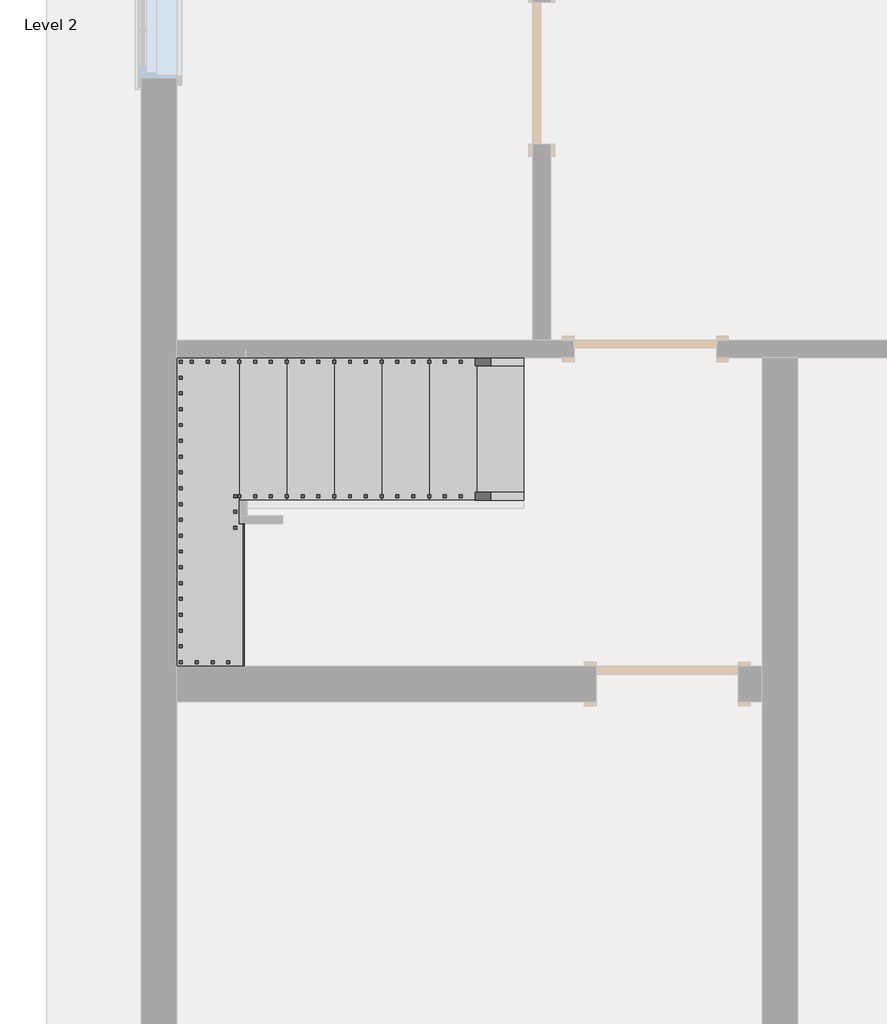
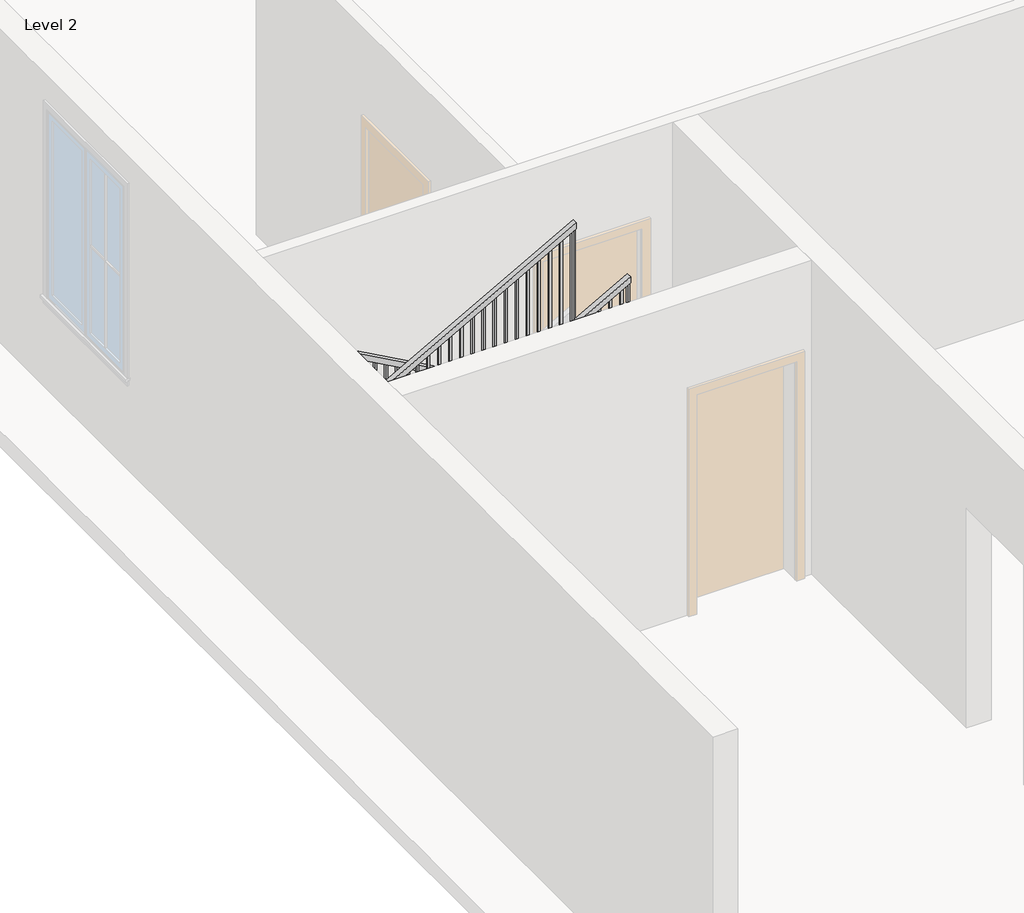
# One storey, part 2 of 3: 2 railings, 1 stair flight.
"""IFC4 building model written with IfcOpenShell, lengths in millimetres."""

from ifc_helpers import new_model, si_unit, frame, origin, place, context, project, spatial, polyline, outline, extrude, faceted_brep, transform, mapped, element, save
from components import stair_flight_2ee17b95

model = new_model("IFC4")

# Units and contexts
model_context = context("Model", 3, world=origin())
ifc_project = project(units=[si_unit("LENGTHUNIT", "METRE", prefix="MILLI")], contexts=[model_context])

# Site, building, storey
site = spatial("IfcSite", under=ifc_project)
building = spatial("IfcBuilding", under=site)
storey = spatial("IfcBuildingStorey", under=building, Name="Level 2", Elevation=3048.0)

# Railings
placement = place(None, origin())
element("IfcRailing", 1, ObjectType="Handrail - Rectangular", at=placement, inside=storey, context=model_context, shape_type="SolidModel", body=[
    faceted_brep([(3727.9146873, 3657.6, 4131.7333333), (3727.9146873, 3657.6, 4073.620221), (3727.9146873, 3708.4, 4073.620221), (3727.9146873, 3708.4, 4131.7333333), (1899.1146873, 3657.6, 5147.7333333), (1885.9510851, 3657.6, 5096.9333333), (1885.9510851, 3708.4, 5096.9333333), (1899.1146873, 3708.4, 5147.7333333), (1549.4, 3657.6, 5147.7333333), (1549.4, 3657.6, 5096.9333333), (1498.6, 3708.4, 5096.9333333), (1498.6, 3708.4, 5147.7333333), (1549.4, 1778.0, 5147.7333333), (1549.4, 1778.0, 5096.9333333), (1498.6, 1727.2, 5096.9333333), (1498.6, 1727.2, 5147.7333333), (1594.3146873, 1778.0, 5147.7333333), (1607.4782895, 1778.0, 5096.9333333), (1607.4782895, 1727.2, 5096.9333333), (1594.3146873, 1727.2, 5147.7333333), (3727.9146873, 1778.0, 6333.0666667), (3727.9146873, 1727.2, 6333.0666667), (3727.9146873, 1727.2, 6274.9535543), (3727.9146873, 1778.0, 6274.9535543)], [[[0, 1, 2, 3]], [[1, 0, 4, 5]], [[2, 1, 5, 6]], [[3, 2, 6, 7]], [[0, 3, 7, 4]], [[5, 4, 8, 9]], [[6, 5, 9, 10]], [[7, 6, 10, 11]], [[4, 7, 11, 8]], [[9, 8, 12, 13]], [[10, 9, 13, 14]], [[11, 10, 14, 15]], [[8, 11, 15, 12]], [[13, 12, 16, 17]], [[14, 13, 17, 18]], [[15, 14, 18, 19]], [[12, 15, 19, 16]], [[20, 21, 22, 23]], [[17, 16, 20, 23]], [[18, 17, 23, 22]], [[19, 18, 22, 21]], [[16, 19, 21, 20]]]),
    extrude(outline(polyline([(6241.1815058, 3667.125), (6230.5981725, 3648.075), (5249.3333333, 3648.075), (5249.3333333, 3667.125), (6241.1815058, 3667.125)])), frame((0.0, 1743.075, 0.0), z_axis=(0.0, 1.0, 0.0), x_axis=(0.0, 0.0, 1.0)), (0.0, 0.0, 1.0), 19.05),
    extrude(outline(polyline([(6184.7370614, 3565.525), (6174.153728, 3546.475), (5249.3333333, 3546.475), (5249.3333333, 3565.525), (6184.7370614, 3565.525)])), frame((0.0, 1743.075, 0.0), z_axis=(0.0, 1.0, 0.0), x_axis=(0.0, 0.0, 1.0)), (0.0, 0.0, 1.0), 19.05),
    extrude(outline(polyline([(6128.2926169, 3463.925), (6117.7092836, 3444.875), (5249.3333333, 3444.875), (5249.3333333, 3463.925), (6128.2926169, 3463.925)])), frame((0.0, 1743.075, 0.0), z_axis=(0.0, 1.0, 0.0), x_axis=(0.0, 0.0, 1.0)), (0.0, 0.0, 1.0), 19.05),
    extrude(outline(polyline([(6071.8481725, 3362.325), (6061.2648391, 3343.275), (5080.0, 3343.275), (5080.0, 3362.325), (6071.8481725, 3362.325)])), frame((0.0, 1743.075, 0.0), z_axis=(0.0, 1.0, 0.0), x_axis=(0.0, 0.0, 1.0)), (0.0, 0.0, 1.0), 19.05),
    extrude(outline(polyline([(6015.403728, 3260.725), (6004.8203947, 3241.675), (5080.0, 3241.675), (5080.0, 3260.725), (6015.403728, 3260.725)])), frame((0.0, 1743.075, 0.0), z_axis=(0.0, 1.0, 0.0), x_axis=(0.0, 0.0, 1.0)), (0.0, 0.0, 1.0), 19.05),
    extrude(outline(polyline([(5958.9592836, 3159.125), (5948.3759503, 3140.075), (5080.0, 3140.075), (5080.0, 3159.125), (5958.9592836, 3159.125)])), frame((0.0, 1743.075, 0.0), z_axis=(0.0, 1.0, 0.0), x_axis=(0.0, 0.0, 1.0)), (0.0, 0.0, 1.0), 19.05),
    extrude(outline(polyline([(5902.5148391, 3057.525), (5891.9315058, 3038.475), (4910.6666667, 3038.475), (4910.6666667, 3057.525), (5902.5148391, 3057.525)])), frame((0.0, 1743.075, 0.0), z_axis=(0.0, 1.0, 0.0), x_axis=(0.0, 0.0, 1.0)), (0.0, 0.0, 1.0), 19.05),
    extrude(outline(polyline([(5846.0703947, 2955.925), (5835.4870614, 2936.875), (4910.6666667, 2936.875), (4910.6666667, 2955.925), (5846.0703947, 2955.925)])), frame((0.0, 1743.075, 0.0), z_axis=(0.0, 1.0, 0.0), x_axis=(0.0, 0.0, 1.0)), (0.0, 0.0, 1.0), 19.05),
    extrude(outline(polyline([(5789.6259503, 2854.325), (5779.0426169, 2835.275), (4910.6666667, 2835.275), (4910.6666667, 2854.325), (5789.6259503, 2854.325)])), frame((0.0, 1743.075, 0.0), z_axis=(0.0, 1.0, 0.0), x_axis=(0.0, 0.0, 1.0)), (0.0, 0.0, 1.0), 19.05),
    extrude(outline(polyline([(5733.1815058, 2752.725), (5722.5981725, 2733.675), (4741.3333333, 2733.675), (4741.3333333, 2752.725), (5733.1815058, 2752.725)])), frame((0.0, 1743.075, 0.0), z_axis=(0.0, 1.0, 0.0), x_axis=(0.0, 0.0, 1.0)), (0.0, 0.0, 1.0), 19.05),
    extrude(outline(polyline([(5676.7370614, 2651.125), (5666.153728, 2632.075), (4741.3333333, 2632.075), (4741.3333333, 2651.125), (5676.7370614, 2651.125)])), frame((0.0, 1743.075, 0.0), z_axis=(0.0, 1.0, 0.0), x_axis=(0.0, 0.0, 1.0)), (0.0, 0.0, 1.0), 19.05),
    extrude(outline(polyline([(5620.2926169, 2549.525), (5609.7092836, 2530.475), (4741.3333333, 2530.475), (4741.3333333, 2549.525), (5620.2926169, 2549.525)])), frame((0.0, 1743.075, 0.0), z_axis=(0.0, 1.0, 0.0), x_axis=(0.0, 0.0, 1.0)), (0.0, 0.0, 1.0), 19.05),
    extrude(outline(polyline([(5563.8481725, 2447.925), (5553.2648391, 2428.875), (4572.0, 2428.875), (4572.0, 2447.925), (5563.8481725, 2447.925)])), frame((0.0, 1743.075, 0.0), z_axis=(0.0, 1.0, 0.0), x_axis=(0.0, 0.0, 1.0)), (0.0, 0.0, 1.0), 19.05),
    extrude(outline(polyline([(5507.403728, 2346.325), (5496.8203947, 2327.275), (4572.0, 2327.275), (4572.0, 2346.325), (5507.403728, 2346.325)])), frame((0.0, 1743.075, 0.0), z_axis=(0.0, 1.0, 0.0), x_axis=(0.0, 0.0, 1.0)), (0.0, 0.0, 1.0), 19.05),
    extrude(outline(polyline([(5450.9592836, 2244.725), (5440.3759503, 2225.675), (4572.0, 2225.675), (4572.0, 2244.725), (5450.9592836, 2244.725)])), frame((0.0, 1743.075, 0.0), z_axis=(0.0, 1.0, 0.0), x_axis=(0.0, 0.0, 1.0)), (0.0, 0.0, 1.0), 19.05),
    extrude(outline(polyline([(5394.5148391, 2143.125), (5383.9315058, 2124.075), (4402.6666667, 2124.075), (4402.6666667, 2143.125), (5394.5148391, 2143.125)])), frame((0.0, 1743.075, 0.0), z_axis=(0.0, 1.0, 0.0), x_axis=(0.0, 0.0, 1.0)), (0.0, 0.0, 1.0), 19.05),
    extrude(outline(polyline([(5338.0703947, 2041.525), (5327.4870614, 2022.475), (4402.6666667, 2022.475), (4402.6666667, 2041.525), (5338.0703947, 2041.525)])), frame((0.0, 1743.075, 0.0), z_axis=(0.0, 1.0, 0.0), x_axis=(0.0, 0.0, 1.0)), (0.0, 0.0, 1.0), 19.05),
    extrude(outline(polyline([(5281.6259503, 1939.925), (5271.0426169, 1920.875), (4402.6666667, 1920.875), (4402.6666667, 1939.925), (5281.6259503, 1939.925)])), frame((0.0, 1743.075, 0.0), z_axis=(0.0, 1.0, 0.0), x_axis=(0.0, 0.0, 1.0)), (0.0, 0.0, 1.0), 19.05),
    extrude(outline(polyline([(5225.1815058, 1838.325), (5214.5981725, 1819.275), (4233.3333333, 1819.275), (4233.3333333, 1838.325), (5225.1815058, 1838.325)])), frame((0.0, 1743.075, 0.0), z_axis=(0.0, 1.0, 0.0), x_axis=(0.0, 0.0, 1.0)), (0.0, 0.0, 1.0), 19.05),
    extrude(outline(polyline([(5168.7370614, 1736.725), (5158.153728, 1717.675), (4233.3333333, 1717.675), (4233.3333333, 1736.725), (5168.7370614, 1736.725)])), frame((0.0, 1743.075, 0.0), z_axis=(0.0, 1.0, 0.0), x_axis=(0.0, 0.0, 1.0)), (0.0, 0.0, 1.0), 19.05),
    extrude(outline(polyline([(5112.2926169, 1635.125), (5101.7092836, 1616.075), (4233.3333333, 1616.075), (4233.3333333, 1635.125), (5112.2926169, 1635.125)])), frame((0.0, 1743.075, 0.0), z_axis=(0.0, 1.0, 0.0), x_axis=(0.0, 0.0, 1.0)), (0.0, 0.0, 1.0), 19.05),
    extrude(outline(polyline([(1514.475, 1863.725), (1533.525, 1863.725), (1533.525, 1844.675), (1514.475, 1844.675), (1514.475, 1863.725)])), frame((0.0, 0.0, 4233.3333333), z_axis=(0.0, 0.0, 1.0), x_axis=(1.0, 0.0, 0.0)), (0.0, 0.0, 1.0), 863.6),
    extrude(outline(polyline([(1514.475, 1965.325), (1533.525, 1965.325), (1533.525, 1946.275), (1514.475, 1946.275), (1514.475, 1965.325)])), frame((0.0, 0.0, 4233.3333333), z_axis=(0.0, 0.0, 1.0), x_axis=(1.0, 0.0, 0.0)), (0.0, 0.0, 1.0), 863.6),
    extrude(outline(polyline([(1514.475, 2066.925), (1533.525, 2066.925), (1533.525, 2047.875), (1514.475, 2047.875), (1514.475, 2066.925)])), frame((0.0, 0.0, 4233.3333333), z_axis=(0.0, 0.0, 1.0), x_axis=(1.0, 0.0, 0.0)), (0.0, 0.0, 1.0), 863.6),
    extrude(outline(polyline([(1514.475, 2168.525), (1533.525, 2168.525), (1533.525, 2149.475), (1514.475, 2149.475), (1514.475, 2168.525)])), frame((0.0, 0.0, 4233.3333333), z_axis=(0.0, 0.0, 1.0), x_axis=(1.0, 0.0, 0.0)), (0.0, 0.0, 1.0), 863.6),
    extrude(outline(polyline([(1514.475, 2270.125), (1533.525, 2270.125), (1533.525, 2251.075), (1514.475, 2251.075), (1514.475, 2270.125)])), frame((0.0, 0.0, 4233.3333333), z_axis=(0.0, 0.0, 1.0), x_axis=(1.0, 0.0, 0.0)), (0.0, 0.0, 1.0), 863.6),
    extrude(outline(polyline([(1514.475, 2371.725), (1533.525, 2371.725), (1533.525, 2352.675), (1514.475, 2352.675), (1514.475, 2371.725)])), frame((0.0, 0.0, 4233.3333333), z_axis=(0.0, 0.0, 1.0), x_axis=(1.0, 0.0, 0.0)), (0.0, 0.0, 1.0), 863.6),
    extrude(outline(polyline([(1514.475, 2473.325), (1533.525, 2473.325), (1533.525, 2454.275), (1514.475, 2454.275), (1514.475, 2473.325)])), frame((0.0, 0.0, 4233.3333333), z_axis=(0.0, 0.0, 1.0), x_axis=(1.0, 0.0, 0.0)), (0.0, 0.0, 1.0), 863.6),
    extrude(outline(polyline([(1514.475, 2574.925), (1533.525, 2574.925), (1533.525, 2555.875), (1514.475, 2555.875), (1514.475, 2574.925)])), frame((0.0, 0.0, 4233.3333333), z_axis=(0.0, 0.0, 1.0), x_axis=(1.0, 0.0, 0.0)), (0.0, 0.0, 1.0), 863.6),
    extrude(outline(polyline([(1514.475, 2676.525), (1533.525, 2676.525), (1533.525, 2657.475), (1514.475, 2657.475), (1514.475, 2676.525)])), frame((0.0, 0.0, 4233.3333333), z_axis=(0.0, 0.0, 1.0), x_axis=(1.0, 0.0, 0.0)), (0.0, 0.0, 1.0), 863.6),
    extrude(outline(polyline([(1514.475, 2778.125), (1533.525, 2778.125), (1533.525, 2759.075), (1514.475, 2759.075), (1514.475, 2778.125)])), frame((0.0, 0.0, 4233.3333333), z_axis=(0.0, 0.0, 1.0), x_axis=(1.0, 0.0, 0.0)), (0.0, 0.0, 1.0), 863.6),
    extrude(outline(polyline([(1514.475, 2879.725), (1533.525, 2879.725), (1533.525, 2860.675), (1514.475, 2860.675), (1514.475, 2879.725)])), frame((0.0, 0.0, 4233.3333333), z_axis=(0.0, 0.0, 1.0), x_axis=(1.0, 0.0, 0.0)), (0.0, 0.0, 1.0), 863.6),
    extrude(outline(polyline([(1514.475, 2981.325), (1533.525, 2981.325), (1533.525, 2962.275), (1514.475, 2962.275), (1514.475, 2981.325)])), frame((0.0, 0.0, 4233.3333333), z_axis=(0.0, 0.0, 1.0), x_axis=(1.0, 0.0, 0.0)), (0.0, 0.0, 1.0), 863.6),
    extrude(outline(polyline([(1514.475, 3082.925), (1533.525, 3082.925), (1533.525, 3063.875), (1514.475, 3063.875), (1514.475, 3082.925)])), frame((0.0, 0.0, 4233.3333333), z_axis=(0.0, 0.0, 1.0), x_axis=(1.0, 0.0, 0.0)), (0.0, 0.0, 1.0), 863.6),
    extrude(outline(polyline([(1514.475, 3184.525), (1533.525, 3184.525), (1533.525, 3165.475), (1514.475, 3165.475), (1514.475, 3184.525)])), frame((0.0, 0.0, 4233.3333333), z_axis=(0.0, 0.0, 1.0), x_axis=(1.0, 0.0, 0.0)), (0.0, 0.0, 1.0), 863.6),
    extrude(outline(polyline([(1514.475, 3286.125), (1533.525, 3286.125), (1533.525, 3267.075), (1514.475, 3267.075), (1514.475, 3286.125)])), frame((0.0, 0.0, 4233.3333333), z_axis=(0.0, 0.0, 1.0), x_axis=(1.0, 0.0, 0.0)), (0.0, 0.0, 1.0), 863.6),
    extrude(outline(polyline([(1514.475, 3387.725), (1533.525, 3387.725), (1533.525, 3368.675), (1514.475, 3368.675), (1514.475, 3387.725)])), frame((0.0, 0.0, 4233.3333333), z_axis=(0.0, 0.0, 1.0), x_axis=(1.0, 0.0, 0.0)), (0.0, 0.0, 1.0), 863.6),
    extrude(outline(polyline([(1514.475, 3489.325), (1533.525, 3489.325), (1533.525, 3470.275), (1514.475, 3470.275), (1514.475, 3489.325)])), frame((0.0, 0.0, 4233.3333333), z_axis=(0.0, 0.0, 1.0), x_axis=(1.0, 0.0, 0.0)), (0.0, 0.0, 1.0), 863.6),
    extrude(outline(polyline([(1514.475, 3590.925), (1533.525, 3590.925), (1533.525, 3571.875), (1514.475, 3571.875), (1514.475, 3590.925)])), frame((0.0, 0.0, 4233.3333333), z_axis=(0.0, 0.0, 1.0), x_axis=(1.0, 0.0, 0.0)), (0.0, 0.0, 1.0), 863.6),
    extrude(outline(polyline([(1603.8396873, 3692.525), (1603.8396873, 3673.475), (1584.7896873, 3673.475), (1584.7896873, 3692.525), (1603.8396873, 3692.525)])), frame((0.0, 0.0, 4233.3333333), z_axis=(0.0, 0.0, 1.0), x_axis=(1.0, 0.0, 0.0)), (0.0, 0.0, 1.0), 863.6),
    extrude(outline(polyline([(1705.4396873, 3692.525), (1705.4396873, 3673.475), (1686.3896873, 3673.475), (1686.3896873, 3692.525), (1705.4396873, 3692.525)])), frame((0.0, 0.0, 4233.3333333), z_axis=(0.0, 0.0, 1.0), x_axis=(1.0, 0.0, 0.0)), (0.0, 0.0, 1.0), 863.6),
    extrude(outline(polyline([(1807.0396873, 3692.525), (1807.0396873, 3673.475), (1787.9896873, 3673.475), (1787.9896873, 3692.525), (1807.0396873, 3692.525)])), frame((0.0, 0.0, 4233.3333333), z_axis=(0.0, 0.0, 1.0), x_axis=(1.0, 0.0, 0.0)), (0.0, 0.0, 1.0), 863.6),
    extrude(outline(polyline([(5084.3285543, 1908.6396873), (5094.9118876, 1889.5896873), (4233.3333333, 1889.5896873), (4233.3333333, 1908.6396873), (5084.3285543, 1908.6396873)])), frame((0.0, 3673.475, 0.0), z_axis=(0.0, 1.0, 0.0), x_axis=(0.0, 0.0, 1.0)), (0.0, 0.0, 1.0), 19.05),
    extrude(outline(polyline([(5027.8841099, 2010.2396873), (5038.4674432, 1991.1896873), (4064.0, 1991.1896873), (4064.0, 2010.2396873), (5027.8841099, 2010.2396873)])), frame((0.0, 3673.475, 0.0), z_axis=(0.0, 1.0, 0.0), x_axis=(0.0, 0.0, 1.0)), (0.0, 0.0, 1.0), 19.05),
    extrude(outline(polyline([(4971.4396654, 2111.8396873), (4982.0229988, 2092.7896873), (4064.0, 2092.7896873), (4064.0, 2111.8396873), (4971.4396654, 2111.8396873)])), frame((0.0, 3673.475, 0.0), z_axis=(0.0, 1.0, 0.0), x_axis=(0.0, 0.0, 1.0)), (0.0, 0.0, 1.0), 19.05),
    extrude(outline(polyline([(4914.995221, 2213.4396873), (4925.5785543, 2194.3896873), (4064.0, 2194.3896873), (4064.0, 2213.4396873), (4914.995221, 2213.4396873)])), frame((0.0, 3673.475, 0.0), z_axis=(0.0, 1.0, 0.0), x_axis=(0.0, 0.0, 1.0)), (0.0, 0.0, 1.0), 19.05),
    extrude(outline(polyline([(4858.5507765, 2315.0396873), (4869.1341099, 2295.9896873), (3894.6666667, 2295.9896873), (3894.6666667, 2315.0396873), (4858.5507765, 2315.0396873)])), frame((0.0, 3673.475, 0.0), z_axis=(0.0, 1.0, 0.0), x_axis=(0.0, 0.0, 1.0)), (0.0, 0.0, 1.0), 19.05),
    extrude(outline(polyline([(4802.1063321, 2416.6396873), (4812.6896654, 2397.5896873), (3894.6666667, 2397.5896873), (3894.6666667, 2416.6396873), (4802.1063321, 2416.6396873)])), frame((0.0, 3673.475, 0.0), z_axis=(0.0, 1.0, 0.0), x_axis=(0.0, 0.0, 1.0)), (0.0, 0.0, 1.0), 19.05),
    extrude(outline(polyline([(4745.6618876, 2518.2396873), (4756.245221, 2499.1896873), (3894.6666667, 2499.1896873), (3894.6666667, 2518.2396873), (4745.6618876, 2518.2396873)])), frame((0.0, 3673.475, 0.0), z_axis=(0.0, 1.0, 0.0), x_axis=(0.0, 0.0, 1.0)), (0.0, 0.0, 1.0), 19.05),
    extrude(outline(polyline([(4689.2174432, 2619.8396873), (4699.8007765, 2600.7896873), (3725.3333333, 2600.7896873), (3725.3333333, 2619.8396873), (4689.2174432, 2619.8396873)])), frame((0.0, 3673.475, 0.0), z_axis=(0.0, 1.0, 0.0), x_axis=(0.0, 0.0, 1.0)), (0.0, 0.0, 1.0), 19.05),
    extrude(outline(polyline([(4632.7729988, 2721.4396873), (4643.3563321, 2702.3896873), (3725.3333333, 2702.3896873), (3725.3333333, 2721.4396873), (4632.7729988, 2721.4396873)])), frame((0.0, 3673.475, 0.0), z_axis=(0.0, 1.0, 0.0), x_axis=(0.0, 0.0, 1.0)), (0.0, 0.0, 1.0), 19.05),
    extrude(outline(polyline([(4576.3285543, 2823.0396873), (4586.9118876, 2803.9896873), (3725.3333333, 2803.9896873), (3725.3333333, 2823.0396873), (4576.3285543, 2823.0396873)])), frame((0.0, 3673.475, 0.0), z_axis=(0.0, 1.0, 0.0), x_axis=(0.0, 0.0, 1.0)), (0.0, 0.0, 1.0), 19.05),
    extrude(outline(polyline([(4519.8841099, 2924.6396873), (4530.4674432, 2905.5896873), (3556.0, 2905.5896873), (3556.0, 2924.6396873), (4519.8841099, 2924.6396873)])), frame((0.0, 3673.475, 0.0), z_axis=(0.0, 1.0, 0.0), x_axis=(0.0, 0.0, 1.0)), (0.0, 0.0, 1.0), 19.05),
    extrude(outline(polyline([(4463.4396654, 3026.2396873), (4474.0229988, 3007.1896873), (3556.0, 3007.1896873), (3556.0, 3026.2396873), (4463.4396654, 3026.2396873)])), frame((0.0, 3673.475, 0.0), z_axis=(0.0, 1.0, 0.0), x_axis=(0.0, 0.0, 1.0)), (0.0, 0.0, 1.0), 19.05),
    extrude(outline(polyline([(4406.995221, 3127.8396873), (4417.5785543, 3108.7896873), (3556.0, 3108.7896873), (3556.0, 3127.8396873), (4406.995221, 3127.8396873)])), frame((0.0, 3673.475, 0.0), z_axis=(0.0, 1.0, 0.0), x_axis=(0.0, 0.0, 1.0)), (0.0, 0.0, 1.0), 19.05),
    extrude(outline(polyline([(4350.5507765, 3229.4396873), (4361.1341099, 3210.3896873), (3386.6666667, 3210.3896873), (3386.6666667, 3229.4396873), (4350.5507765, 3229.4396873)])), frame((0.0, 3673.475, 0.0), z_axis=(0.0, 1.0, 0.0), x_axis=(0.0, 0.0, 1.0)), (0.0, 0.0, 1.0), 19.05),
    extrude(outline(polyline([(4294.1063321, 3331.0396873), (4304.6896654, 3311.9896873), (3386.6666667, 3311.9896873), (3386.6666667, 3331.0396873), (4294.1063321, 3331.0396873)])), frame((0.0, 3673.475, 0.0), z_axis=(0.0, 1.0, 0.0), x_axis=(0.0, 0.0, 1.0)), (0.0, 0.0, 1.0), 19.05),
    extrude(outline(polyline([(4237.6618876, 3432.6396873), (4248.245221, 3413.5896873), (3386.6666667, 3413.5896873), (3386.6666667, 3432.6396873), (4237.6618876, 3432.6396873)])), frame((0.0, 3673.475, 0.0), z_axis=(0.0, 1.0, 0.0), x_axis=(0.0, 0.0, 1.0)), (0.0, 0.0, 1.0), 19.05),
    extrude(outline(polyline([(4181.2174432, 3534.2396873), (4191.8007765, 3515.1896873), (3217.3333333, 3515.1896873), (3217.3333333, 3534.2396873), (4181.2174432, 3534.2396873)])), frame((0.0, 3673.475, 0.0), z_axis=(0.0, 1.0, 0.0), x_axis=(0.0, 0.0, 1.0)), (0.0, 0.0, 1.0), 19.05),
    extrude(outline(polyline([(4124.7729988, 3635.8396873), (4135.3563321, 3616.7896873), (3217.3333333, 3616.7896873), (3217.3333333, 3635.8396873), (4124.7729988, 3635.8396873)])), frame((0.0, 3673.475, 0.0), z_axis=(0.0, 1.0, 0.0), x_axis=(0.0, 0.0, 1.0)), (0.0, 0.0, 1.0), 19.05),
    extrude(outline(polyline([(1514.475, 1762.125), (1533.525, 1762.125), (1533.525, 1743.075), (1514.475, 1743.075), (1514.475, 1762.125)])), frame((0.0, 0.0, 4233.3333333), z_axis=(0.0, 0.0, 1.0), x_axis=(1.0, 0.0, 0.0)), (0.0, 0.0, 1.0), 863.6),
    extrude(outline(polyline([(1533.525, 3692.525), (1533.525, 3673.475), (1514.475, 3673.475), (1514.475, 3692.525), (1533.525, 3692.525)])), frame((0.0, 0.0, 4233.3333333), z_axis=(0.0, 0.0, 1.0), x_axis=(1.0, 0.0, 0.0)), (0.0, 0.0, 1.0), 863.6),
    extrude(outline(polyline([(6274.9535543, 3727.9146873), (6264.370221, 3708.8646873), (5249.3333333, 3708.8646873), (5249.3333333, 3727.9146873), (6274.9535543, 3727.9146873)])), frame((0.0, 1743.075, 0.0), z_axis=(0.0, 1.0, 0.0), x_axis=(0.0, 0.0, 1.0)), (0.0, 0.0, 1.0), 19.05),
    extrude(outline(polyline([(4073.620221, 3727.9146873), (4084.2035543, 3708.8646873), (3217.3333333, 3708.8646873), (3217.3333333, 3727.9146873), (4073.620221, 3727.9146873)])), frame((0.0, 3673.475, 0.0), z_axis=(0.0, 1.0, 0.0), x_axis=(0.0, 0.0, 1.0)), (0.0, 0.0, 1.0), 19.05),
])
element("IfcRailing", 2, ObjectType="Handrail - Rectangular", at=placement, inside=storey, context=model_context, shape_type="SolidModel", body=[
    faceted_brep([(3727.9146873, 2794.0, 4131.7333333), (3727.9146873, 2794.0, 4073.620221), (3727.9146873, 2844.8, 4073.620221), (3727.9146873, 2844.8, 4131.7333333), (1975.3146873, 2794.0, 5105.4), (1924.5146873, 2794.0, 5075.5091099), (1924.5146873, 2844.8, 5075.5091099), (1975.3146873, 2844.8, 5105.4), (1975.3146873, 2794.0, 5147.7333333), (1924.5146873, 2794.0, 5096.9333333), (1924.5146873, 2844.8, 5096.9333333), (1975.3146873, 2844.8, 5147.7333333), (1899.1146873, 2794.0, 5147.7333333), (1899.1146873, 2794.0, 5096.9333333), (1848.3146873, 2844.8, 5096.9333333), (1848.3146873, 2844.8, 5147.7333333), (1899.1146873, 2717.8, 5147.7333333), (1899.1146873, 2667.0, 5096.9333333), (1848.3146873, 2667.0, 5096.9333333), (1848.3146873, 2717.8, 5147.7333333), (1899.1146873, 2717.8, 5359.4), (1899.1146873, 2667.0, 5308.6), (1848.3146873, 2667.0, 5308.6), (1848.3146873, 2717.8, 5359.4), (1899.1146873, 2641.6, 5359.4), (1899.1146873, 2641.6, 5308.6), (1848.3146873, 2590.8, 5308.6), (1848.3146873, 2590.8, 5359.4), (1975.3146873, 2641.6, 5359.4), (1988.4782895, 2641.6, 5308.6), (1988.4782895, 2590.8, 5308.6), (1975.3146873, 2590.8, 5359.4), (3727.9146873, 2641.6, 6333.0666667), (3727.9146873, 2590.8, 6333.0666667), (3727.9146873, 2590.8, 6274.9535543), (3727.9146873, 2641.6, 6274.9535543)], [[[0, 1, 2, 3]], [[1, 0, 4, 5]], [[2, 1, 5, 6]], [[3, 2, 6, 7]], [[0, 3, 7, 4]], [[5, 4, 8, 9]], [[6, 5, 9, 10]], [[7, 6, 10, 11]], [[4, 7, 11, 8]], [[9, 8, 12, 13]], [[10, 9, 13, 14]], [[11, 10, 14, 15]], [[8, 11, 15, 12]], [[13, 12, 16, 17]], [[14, 13, 17, 18]], [[15, 14, 18, 19]], [[12, 15, 19, 16]], [[17, 16, 20, 21]], [[18, 17, 21, 22]], [[19, 18, 22, 23]], [[16, 19, 23, 20]], [[21, 20, 24, 25]], [[22, 21, 25, 26]], [[23, 22, 26, 27]], [[20, 23, 27, 24]], [[25, 24, 28, 29]], [[26, 25, 29, 30]], [[27, 26, 30, 31]], [[24, 27, 31, 28]], [[32, 33, 34, 35]], [[29, 28, 32, 35]], [[30, 29, 35, 34]], [[31, 30, 34, 33]], [[28, 31, 33, 32]]]),
    extrude(outline(polyline([(6255.5507765, 3692.9896873), (5249.3333333, 3692.9896873), (5249.3333333, 3712.0396873), (6266.1341099, 3712.0396873), (6255.5507765, 3692.9896873)])), frame((0.0, 2606.675, 0.0), z_axis=(0.0, 1.0, 0.0), x_axis=(0.0, 0.0, 1.0)), (0.0, 0.0, 1.0), 19.05),
    extrude(outline(polyline([(6199.1063321, 3591.3896873), (5249.3333333, 3591.3896873), (5249.3333333, 3610.4396873), (6209.6896654, 3610.4396873), (6199.1063321, 3591.3896873)])), frame((0.0, 2606.675, 0.0), z_axis=(0.0, 1.0, 0.0), x_axis=(0.0, 0.0, 1.0)), (0.0, 0.0, 1.0), 19.05),
    extrude(outline(polyline([(6142.6618876, 3489.7896873), (5249.3333333, 3489.7896873), (5249.3333333, 3508.8396873), (6153.245221, 3508.8396873), (6142.6618876, 3489.7896873)])), frame((0.0, 2606.675, 0.0), z_axis=(0.0, 1.0, 0.0), x_axis=(0.0, 0.0, 1.0)), (0.0, 0.0, 1.0), 19.05),
    extrude(outline(polyline([(6086.2174432, 3388.1896873), (5080.0, 3388.1896873), (5080.0, 3407.2396873), (6096.8007765, 3407.2396873), (6086.2174432, 3388.1896873)])), frame((0.0, 2606.675, 0.0), z_axis=(0.0, 1.0, 0.0), x_axis=(0.0, 0.0, 1.0)), (0.0, 0.0, 1.0), 19.05),
    extrude(outline(polyline([(6029.7729988, 3286.5896873), (5080.0, 3286.5896873), (5080.0, 3305.6396873), (6040.3563321, 3305.6396873), (6029.7729988, 3286.5896873)])), frame((0.0, 2606.675, 0.0), z_axis=(0.0, 1.0, 0.0), x_axis=(0.0, 0.0, 1.0)), (0.0, 0.0, 1.0), 19.05),
    extrude(outline(polyline([(5973.3285543, 3184.9896873), (5080.0, 3184.9896873), (5080.0, 3204.0396873), (5983.9118876, 3204.0396873), (5973.3285543, 3184.9896873)])), frame((0.0, 2606.675, 0.0), z_axis=(0.0, 1.0, 0.0), x_axis=(0.0, 0.0, 1.0)), (0.0, 0.0, 1.0), 19.05),
    extrude(outline(polyline([(5916.8841099, 3083.3896873), (4910.6666667, 3083.3896873), (4910.6666667, 3102.4396873), (5927.4674432, 3102.4396873), (5916.8841099, 3083.3896873)])), frame((0.0, 2606.675, 0.0), z_axis=(0.0, 1.0, 0.0), x_axis=(0.0, 0.0, 1.0)), (0.0, 0.0, 1.0), 19.05),
    extrude(outline(polyline([(5860.4396654, 2981.7896873), (4910.6666667, 2981.7896873), (4910.6666667, 3000.8396873), (5871.0229988, 3000.8396873), (5860.4396654, 2981.7896873)])), frame((0.0, 2606.675, 0.0), z_axis=(0.0, 1.0, 0.0), x_axis=(0.0, 0.0, 1.0)), (0.0, 0.0, 1.0), 19.05),
    extrude(outline(polyline([(5803.995221, 2880.1896873), (4910.6666667, 2880.1896873), (4910.6666667, 2899.2396873), (5814.5785543, 2899.2396873), (5803.995221, 2880.1896873)])), frame((0.0, 2606.675, 0.0), z_axis=(0.0, 1.0, 0.0), x_axis=(0.0, 0.0, 1.0)), (0.0, 0.0, 1.0), 19.05),
    extrude(outline(polyline([(5747.5507765, 2778.5896873), (4741.3333333, 2778.5896873), (4741.3333333, 2797.6396873), (5758.1341099, 2797.6396873), (5747.5507765, 2778.5896873)])), frame((0.0, 2606.675, 0.0), z_axis=(0.0, 1.0, 0.0), x_axis=(0.0, 0.0, 1.0)), (0.0, 0.0, 1.0), 19.05),
    extrude(outline(polyline([(5691.1063321, 2676.9896873), (4741.3333333, 2676.9896873), (4741.3333333, 2696.0396873), (5701.6896654, 2696.0396873), (5691.1063321, 2676.9896873)])), frame((0.0, 2606.675, 0.0), z_axis=(0.0, 1.0, 0.0), x_axis=(0.0, 0.0, 1.0)), (0.0, 0.0, 1.0), 19.05),
    extrude(outline(polyline([(5634.6618876, 2575.3896873), (4741.3333333, 2575.3896873), (4741.3333333, 2594.4396873), (5645.245221, 2594.4396873), (5634.6618876, 2575.3896873)])), frame((0.0, 2606.675, 0.0), z_axis=(0.0, 1.0, 0.0), x_axis=(0.0, 0.0, 1.0)), (0.0, 0.0, 1.0), 19.05),
    extrude(outline(polyline([(5578.2174432, 2473.7896873), (4572.0, 2473.7896873), (4572.0, 2492.8396873), (5588.8007765, 2492.8396873), (5578.2174432, 2473.7896873)])), frame((0.0, 2606.675, 0.0), z_axis=(0.0, 1.0, 0.0), x_axis=(0.0, 0.0, 1.0)), (0.0, 0.0, 1.0), 19.05),
    extrude(outline(polyline([(5521.7729988, 2372.1896873), (4572.0, 2372.1896873), (4572.0, 2391.2396873), (5532.3563321, 2391.2396873), (5521.7729988, 2372.1896873)])), frame((0.0, 2606.675, 0.0), z_axis=(0.0, 1.0, 0.0), x_axis=(0.0, 0.0, 1.0)), (0.0, 0.0, 1.0), 19.05),
    extrude(outline(polyline([(5465.3285543, 2270.5896873), (4572.0, 2270.5896873), (4572.0, 2289.6396873), (5475.9118876, 2289.6396873), (5465.3285543, 2270.5896873)])), frame((0.0, 2606.675, 0.0), z_axis=(0.0, 1.0, 0.0), x_axis=(0.0, 0.0, 1.0)), (0.0, 0.0, 1.0), 19.05),
    extrude(outline(polyline([(5408.8841099, 2168.9896873), (4402.6666667, 2168.9896873), (4402.6666667, 2188.0396873), (5419.4674432, 2188.0396873), (5408.8841099, 2168.9896873)])), frame((0.0, 2606.675, 0.0), z_axis=(0.0, 1.0, 0.0), x_axis=(0.0, 0.0, 1.0)), (0.0, 0.0, 1.0), 19.05),
    extrude(outline(polyline([(5352.4396654, 2067.3896873), (4402.6666667, 2067.3896873), (4402.6666667, 2086.4396873), (5363.0229988, 2086.4396873), (5352.4396654, 2067.3896873)])), frame((0.0, 2606.675, 0.0), z_axis=(0.0, 1.0, 0.0), x_axis=(0.0, 0.0, 1.0)), (0.0, 0.0, 1.0), 19.05),
    extrude(outline(polyline([(5295.995221, 1965.7896873), (4402.6666667, 1965.7896873), (4402.6666667, 1984.8396873), (5306.5785543, 1984.8396873), (5295.995221, 1965.7896873)])), frame((0.0, 2606.675, 0.0), z_axis=(0.0, 1.0, 0.0), x_axis=(0.0, 0.0, 1.0)), (0.0, 0.0, 1.0), 19.05),
    extrude(outline(polyline([(1883.2396873, 2727.325), (1883.2396873, 2708.275), (1864.1896873, 2708.275), (1864.1896873, 2727.325), (1883.2396873, 2727.325)])), frame((0.0, 0.0, 4233.3333333), z_axis=(0.0, 0.0, 1.0), x_axis=(1.0, 0.0, 0.0)), (0.0, 0.0, 1.0), 863.6),
    extrude(outline(polyline([(1908.6396873, 2809.875), (1889.5896873, 2809.875), (1889.5896873, 2828.925), (1908.6396873, 2828.925), (1908.6396873, 2809.875)])), frame((0.0, 0.0, 4233.3333333), z_axis=(0.0, 0.0, 1.0), x_axis=(1.0, 0.0, 0.0)), (0.0, 0.0, 1.0), 863.6),
    extrude(outline(polyline([(5038.4674432, 1991.1896873), (4064.0, 1991.1896873), (4064.0, 2010.2396873), (5027.8841099, 2010.2396873), (5038.4674432, 1991.1896873)])), frame((0.0, 2809.875, 0.0), z_axis=(0.0, 1.0, 0.0), x_axis=(0.0, 0.0, 1.0)), (0.0, 0.0, 1.0), 19.05),
    extrude(outline(polyline([(4982.0229988, 2092.7896873), (4064.0, 2092.7896873), (4064.0, 2111.8396873), (4971.4396654, 2111.8396873), (4982.0229988, 2092.7896873)])), frame((0.0, 2809.875, 0.0), z_axis=(0.0, 1.0, 0.0), x_axis=(0.0, 0.0, 1.0)), (0.0, 0.0, 1.0), 19.05),
    extrude(outline(polyline([(4925.5785543, 2194.3896873), (4064.0, 2194.3896873), (4064.0, 2213.4396873), (4914.995221, 2213.4396873), (4925.5785543, 2194.3896873)])), frame((0.0, 2809.875, 0.0), z_axis=(0.0, 1.0, 0.0), x_axis=(0.0, 0.0, 1.0)), (0.0, 0.0, 1.0), 19.05),
    extrude(outline(polyline([(4869.1341099, 2295.9896873), (3894.6666667, 2295.9896873), (3894.6666667, 2315.0396873), (4858.5507765, 2315.0396873), (4869.1341099, 2295.9896873)])), frame((0.0, 2809.875, 0.0), z_axis=(0.0, 1.0, 0.0), x_axis=(0.0, 0.0, 1.0)), (0.0, 0.0, 1.0), 19.05),
    extrude(outline(polyline([(4812.6896654, 2397.5896873), (3894.6666667, 2397.5896873), (3894.6666667, 2416.6396873), (4802.1063321, 2416.6396873), (4812.6896654, 2397.5896873)])), frame((0.0, 2809.875, 0.0), z_axis=(0.0, 1.0, 0.0), x_axis=(0.0, 0.0, 1.0)), (0.0, 0.0, 1.0), 19.05),
    extrude(outline(polyline([(4756.245221, 2499.1896873), (3894.6666667, 2499.1896873), (3894.6666667, 2518.2396873), (4745.6618876, 2518.2396873), (4756.245221, 2499.1896873)])), frame((0.0, 2809.875, 0.0), z_axis=(0.0, 1.0, 0.0), x_axis=(0.0, 0.0, 1.0)), (0.0, 0.0, 1.0), 19.05),
    extrude(outline(polyline([(4699.8007765, 2600.7896873), (3725.3333333, 2600.7896873), (3725.3333333, 2619.8396873), (4689.2174432, 2619.8396873), (4699.8007765, 2600.7896873)])), frame((0.0, 2809.875, 0.0), z_axis=(0.0, 1.0, 0.0), x_axis=(0.0, 0.0, 1.0)), (0.0, 0.0, 1.0), 19.05),
    extrude(outline(polyline([(4643.3563321, 2702.3896873), (3725.3333333, 2702.3896873), (3725.3333333, 2721.4396873), (4632.7729988, 2721.4396873), (4643.3563321, 2702.3896873)])), frame((0.0, 2809.875, 0.0), z_axis=(0.0, 1.0, 0.0), x_axis=(0.0, 0.0, 1.0)), (0.0, 0.0, 1.0), 19.05),
    extrude(outline(polyline([(4586.9118876, 2803.9896873), (3725.3333333, 2803.9896873), (3725.3333333, 2823.0396873), (4576.3285543, 2823.0396873), (4586.9118876, 2803.9896873)])), frame((0.0, 2809.875, 0.0), z_axis=(0.0, 1.0, 0.0), x_axis=(0.0, 0.0, 1.0)), (0.0, 0.0, 1.0), 19.05),
    extrude(outline(polyline([(4530.4674432, 2905.5896873), (3556.0, 2905.5896873), (3556.0, 2924.6396873), (4519.8841099, 2924.6396873), (4530.4674432, 2905.5896873)])), frame((0.0, 2809.875, 0.0), z_axis=(0.0, 1.0, 0.0), x_axis=(0.0, 0.0, 1.0)), (0.0, 0.0, 1.0), 19.05),
    extrude(outline(polyline([(4474.0229988, 3007.1896873), (3556.0, 3007.1896873), (3556.0, 3026.2396873), (4463.4396654, 3026.2396873), (4474.0229988, 3007.1896873)])), frame((0.0, 2809.875, 0.0), z_axis=(0.0, 1.0, 0.0), x_axis=(0.0, 0.0, 1.0)), (0.0, 0.0, 1.0), 19.05),
    extrude(outline(polyline([(4417.5785543, 3108.7896873), (3556.0, 3108.7896873), (3556.0, 3127.8396873), (4406.995221, 3127.8396873), (4417.5785543, 3108.7896873)])), frame((0.0, 2809.875, 0.0), z_axis=(0.0, 1.0, 0.0), x_axis=(0.0, 0.0, 1.0)), (0.0, 0.0, 1.0), 19.05),
    extrude(outline(polyline([(4361.1341099, 3210.3896873), (3386.6666667, 3210.3896873), (3386.6666667, 3229.4396873), (4350.5507765, 3229.4396873), (4361.1341099, 3210.3896873)])), frame((0.0, 2809.875, 0.0), z_axis=(0.0, 1.0, 0.0), x_axis=(0.0, 0.0, 1.0)), (0.0, 0.0, 1.0), 19.05),
    extrude(outline(polyline([(4304.6896654, 3311.9896873), (3386.6666667, 3311.9896873), (3386.6666667, 3331.0396873), (4294.1063321, 3331.0396873), (4304.6896654, 3311.9896873)])), frame((0.0, 2809.875, 0.0), z_axis=(0.0, 1.0, 0.0), x_axis=(0.0, 0.0, 1.0)), (0.0, 0.0, 1.0), 19.05),
    extrude(outline(polyline([(4248.245221, 3413.5896873), (3386.6666667, 3413.5896873), (3386.6666667, 3432.6396873), (4237.6618876, 3432.6396873), (4248.245221, 3413.5896873)])), frame((0.0, 2809.875, 0.0), z_axis=(0.0, 1.0, 0.0), x_axis=(0.0, 0.0, 1.0)), (0.0, 0.0, 1.0), 19.05),
    extrude(outline(polyline([(4191.8007765, 3515.1896873), (3217.3333333, 3515.1896873), (3217.3333333, 3534.2396873), (4181.2174432, 3534.2396873), (4191.8007765, 3515.1896873)])), frame((0.0, 2809.875, 0.0), z_axis=(0.0, 1.0, 0.0), x_axis=(0.0, 0.0, 1.0)), (0.0, 0.0, 1.0), 19.05),
    extrude(outline(polyline([(4135.3563321, 3616.7896873), (3217.3333333, 3616.7896873), (3217.3333333, 3635.8396873), (4124.7729988, 3635.8396873), (4135.3563321, 3616.7896873)])), frame((0.0, 2809.875, 0.0), z_axis=(0.0, 1.0, 0.0), x_axis=(0.0, 0.0, 1.0)), (0.0, 0.0, 1.0), 19.05),
    extrude(outline(polyline([(1883.2396873, 2625.725), (1883.2396873, 2606.675), (1864.1896873, 2606.675), (1864.1896873, 2625.725), (1883.2396873, 2625.725)])), frame((0.0, 0.0, 4233.3333333), z_axis=(0.0, 0.0, 1.0), x_axis=(1.0, 0.0, 0.0)), (0.0, 0.0, 1.0), 1075.2666667),
    extrude(outline(polyline([(1883.2396873, 2809.875), (1864.1896873, 2809.875), (1864.1896873, 2828.925), (1883.2396873, 2828.925), (1883.2396873, 2809.875)])), frame((0.0, 0.0, 4233.3333333), z_axis=(0.0, 0.0, 1.0), x_axis=(1.0, 0.0, 0.0)), (0.0, 0.0, 1.0), 863.6),
    extrude(outline(polyline([(6264.370221, 3708.8646873), (5249.3333333, 3708.8646873), (5249.3333333, 3727.9146873), (6274.9535543, 3727.9146873), (6264.370221, 3708.8646873)])), frame((0.0, 2606.675, 0.0), z_axis=(0.0, 1.0, 0.0), x_axis=(0.0, 0.0, 1.0)), (0.0, 0.0, 1.0), 19.05),
    extrude(outline(polyline([(4084.2035543, 3708.8646873), (3217.3333333, 3708.8646873), (3217.3333333, 3727.9146873), (4073.620221, 3727.9146873), (4084.2035543, 3708.8646873)])), frame((0.0, 2809.875, 0.0), z_axis=(0.0, 1.0, 0.0), x_axis=(0.0, 0.0, 1.0)), (0.0, 0.0, 1.0), 19.05),
])

# Stair flight
stair_flight_shape = stair_flight_2ee17b95(model_context)
element("IfcStairFlight", 3, ObjectType="2\" Tread 1\" Nosing 1/4\" Riser", at=placement, inside=storey, context=model_context, shape_type="MappedRepresentation", body=[
    mapped(stair_flight_shape, transform((0.0, 0.0, 0.0), x_axis=(1.0, 0.0, 0.0), y_axis=(0.0, 1.0, 0.0), z_axis=(0.0, 0.0, 1.0))),
])

save(model, "model.ifc")

# Revit data of these elements
# Type "Handrail - Rectangular"
#   Assembly Code = "C2010400"
#   built-in parameter 1008612 = 0.0416667 (stored number, unit not read)
#   built-in parameter 1008611 = 0.0416667 (stored number, unit not read)
#   built-in parameter 1008609 = 0.333333 (stored number, unit not read)
#   built-in parameter 1008604 = 0.166667 (stored number, unit not read)
#   built-in parameter 1008603 = 0.166667 (stored number, unit not read)
#   Railing Height = 3' - 0"
#   built-in parameter 1008630 = 2
#   built-in parameter 1008610 = 2
#   built-in parameter 1008618 = Baluster - Square : 3/4"
# Elements 1, 2 (IfcRailing, "Handrail - Rectangular")
#   Phase Created = New Construction
# Element 3 (IfcStairFlight, "2\" Tread 1\" Nosing 1/4\" Riser")
#   Phase Created = New Construction
